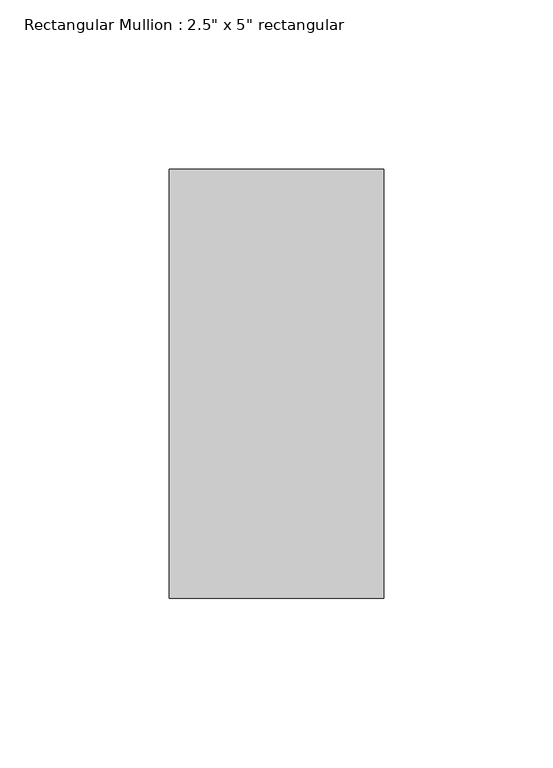
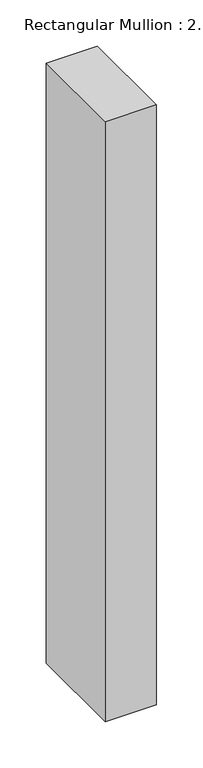
"""IFC4 building model written with IfcOpenShell, lengths in millimetres: member geometry."""

from ifc_helpers import new_model, si_unit, frame, origin, place, context, project, spatial, polyline, outline, extrude, source, transform, mapped, element, save


def member_c3a135b3(model_context):
    return source(origin(), model_context, "Body", "SweptSolid", [
        extrude(outline(polyline([(0.0, 63.5), (0.0, -63.5), (-63.5, -63.5), (-63.5, 63.5), (0.0, 63.5)])), frame((0.0, 0.0, -788.6592248), z_axis=(0.0, 0.0, 1.0), x_axis=(1.0, 0.0, 0.0)), (0.0, 0.0, 1.0), 788.6592248),
    ])


if __name__ == "__main__":
    model = new_model("IFC4")
    model_context = context("Model", 3, world=origin())
    ifc_project = project(units=[si_unit("LENGTHUNIT", "METRE", prefix="MILLI")], contexts=[model_context])
    site = spatial("IfcSite", under=ifc_project)
    building = spatial("IfcBuilding", under=site)
    placement = place(None, origin())
    member_shape = member_c3a135b3(model_context)
    element("IfcMember", 1, ObjectType="Rectangular Mullion : 2.5\" x 5\" rectangular", at=placement, inside=building, context=model_context, shape_type="MappedRepresentation", body=[
        mapped(member_shape, transform((0.0, 0.0, 0.0), x_axis=(1.0, 0.0, 0.0), y_axis=(0.0, 1.0, 0.0), z_axis=(0.0, 0.0, 1.0))),
    ])
    save(model, "model.ifc")

# Revit data of these elements
# Type "Rectangular Mullion : 2.5\" x 5\" rectangular"
#   built-in parameter 1007304 = 0.416667 (stored number, unit not read)
#   built-in parameter 1007301 = 0.104167 (stored number, unit not read)
#   built-in parameter 1007300 = 0.104167 (stored number, unit not read)
# Element 1 (IfcMember, "Rectangular Mullion : 2.5\" x 5\" rectangular")
#   Materials on its faces: "Roofing, EPDM Membrane"
# Materials
#   "Roofing, EPDM Membrane": class "Generic", colour RGB 127 127 127, transparency 0, Description = "EPDM roof membrane", Cost = 0
